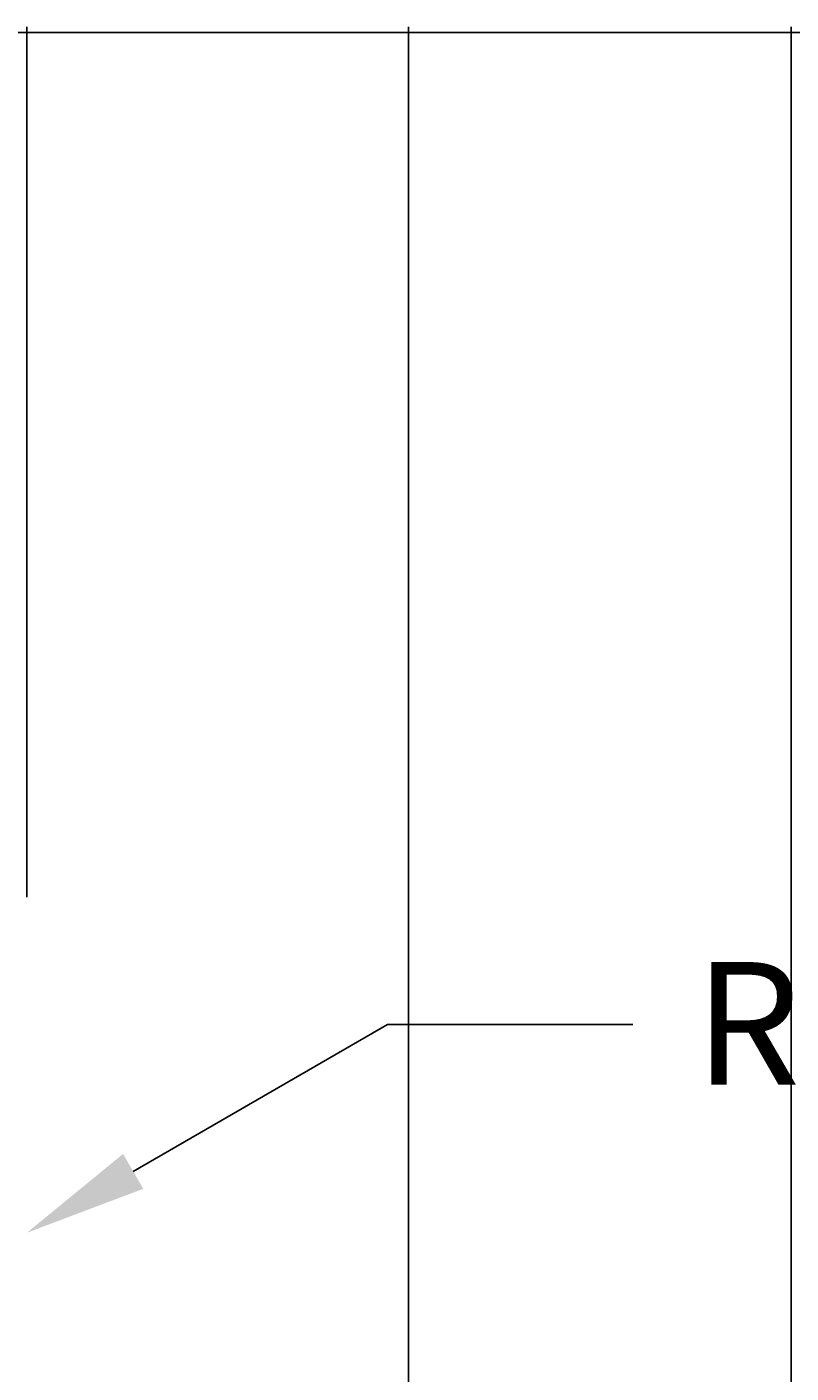
# Model space of a CAD drawing. Units: millimetres. Extents: x -11 to 280, y -4 to 208.
# Tile 18 of 55: x 66 to 91, y 164 to 208. Entities that reach past the tile are written whole.
import ezdxf
from ezdxf import colors
from ezdxf.entities.mleader import LeaderData, LeaderLine
from ezdxf.math import Vec2, Vec3

# ---------------------------------------------------------------- set-up
doc = ezdxf.new("R2010")
doc.units = ezdxf.units.MM
doc.layers.add('M-ANNO-TEXT', color=7, linetype='Continuous', lineweight=18)
doc.layers.add('M-DIMS', color=2, linetype='Continuous', lineweight=18)
doc.styles.get("Standard").update_dxf_attribs({"font": 'arial.ttf'})
doc.dimstyles.get("Standard").update_dxf_attribs({"dimtxt": 0.18, "dimasz": 0.18, "dimexe": 0.18, "dimexo": 0.0625, "dimgap": 0.09, "dimtad": 0, "dimtih": 1, "dimtoh": 1, "dimdec": 4, "dimzin": 0, "dimdsep": 46, "dimtxsty": 'Standard', "dimcen": 0.09, "dimadec": 0, "dimazin": 0, "dimtfac": 1, "dimtdec": 4, "dimtofl": 0, "dimtmove": 0, "dimatfit": 3, "dimfxl": 1, "dimtolj": 1, "dimtzin": 0, "dimarcsym": 0})

# ---------------------------------------------------------------- blocks, each defined once
blk = doc.blocks.new('*D5')
at = {"layer": 'Defpoints', "color": 0, "transparency": 16777216}
for p in [(24.759, 192.645), (-10.087, 11.435), (261.686, 11.435)]:
    blk.add_point(p, dxfattribs=at)
at = {"layer": 'M-DIMS', "color": 0, "lineweight": -2, "transparency": 16777216}
for p, q in [((24.696, 192.645), (-10.267, 192.645)), ((-10.087, 192.465), (-10.087, 102.222)), ((-10.087, 11.615), (-10.087, 101.858)), ((261.624, 11.435), (-10.267, 11.435))]:
    blk.add_line(p, q, dxfattribs=at)
at = {"layer": 'M-DIMS', "color": 0, "transparency": 16777216}
for points in [[(-10.117, 192.465), (-10.057, 192.465), (-10.087, 192.645)], [(-10.117, 11.615), (-10.057, 11.615), (-10.087, 11.435)]]:
    blk.add_solid(points, dxfattribs=at)
at = {"layer": 'M-DIMS', "color": 0, "transparency": 16777216, "insert": (-10.087, 102.04), "char_height": 0.18, "attachment_point": 5}
blk.add_mtext('\\A1;181.2', dxfattribs=at)
blk = doc.blocks.new('*D6')
at = {"layer": 'Defpoints', "color": 0, "transparency": 16777216}
for p in [(236.935, 207.495), (66.388, 179.241), (236.935, 165.103)]:
    blk.add_point(p, dxfattribs=at)
at = {"layer": 'M-DIMS', "color": 0, "lineweight": -2, "transparency": 16777216}
for p, q in [((66.388, 179.304), (66.388, 207.675)), ((236.935, 165.166), (236.935, 207.675)), ((66.568, 207.495), (151.206, 207.495)), ((236.755, 207.495), (152.117, 207.495))]:
    blk.add_line(p, q, dxfattribs=at)
at = {"layer": 'M-DIMS', "color": 0, "transparency": 16777216}
for points in [[(66.568, 207.525), (66.568, 207.465), (66.388, 207.495)], [(236.755, 207.525), (236.755, 207.465), (236.935, 207.495)]]:
    blk.add_solid(points, dxfattribs=at)
at = {"layer": 'M-DIMS', "color": 0, "transparency": 16777216, "insert": (151.661, 207.495), "char_height": 0.18, "attachment_point": 5}
blk.add_mtext('\\A1;170.55', dxfattribs=at)
blk = doc.blocks.new('*D9')
at = {"layer": 'Defpoints', "color": 0, "transparency": 16777216}
for p in [(78.827, 207.495), (31.006, 98.021), (78.827, 98.149)]:
    blk.add_point(p, dxfattribs=at)
at = {"layer": 'M-DIMS', "color": 0, "lineweight": -2, "transparency": 16777216}
for p, q in [((31.006, 98.084), (31.006, 207.675)), ((78.827, 98.212), (78.827, 207.675)), ((31.186, 207.495), (54.52, 207.495)), ((78.647, 207.495), (55.313, 207.495))]:
    blk.add_line(p, q, dxfattribs=at)
at = {"layer": 'M-DIMS', "color": 0, "transparency": 16777216}
for points in [[(31.186, 207.525), (31.186, 207.465), (31.006, 207.495)], [(78.647, 207.525), (78.647, 207.465), (78.827, 207.495)]]:
    blk.add_solid(points, dxfattribs=at)
at = {"layer": 'M-DIMS', "color": 0, "transparency": 16777216, "insert": (54.917, 207.495), "char_height": 0.18, "attachment_point": 5}
blk.add_mtext('\\A1;47.82', dxfattribs=at)
blk = doc.blocks.new('*D11')
at = {"layer": 'Defpoints', "color": 0, "transparency": 16777216}
for p in [(118.514, 207.495), (91.3, 98.149), (118.514, 96.485)]:
    blk.add_point(p, dxfattribs=at)
at = {"layer": 'M-DIMS', "color": 0, "lineweight": -2, "transparency": 16777216}
for p, q in [((91.3, 98.212), (91.3, 207.675)), ((118.514, 96.547), (118.514, 207.675)), ((91.48, 207.495), (104.442, 207.495)), ((118.334, 207.495), (105.372, 207.495))]:
    blk.add_line(p, q, dxfattribs=at)
at = {"layer": 'M-DIMS', "color": 0, "transparency": 16777216}
for points in [[(91.48, 207.525), (91.48, 207.465), (91.3, 207.495)], [(118.334, 207.525), (118.334, 207.465), (118.514, 207.495)]]:
    blk.add_solid(points, dxfattribs=at)
at = {"layer": 'M-DIMS', "color": 0, "transparency": 16777216, "insert": (104.907, 207.495), "char_height": 0.18, "attachment_point": 5}
blk.add_mtext('\\A1;27.214', dxfattribs=at)

msp = doc.modelspace()

# ---------------------------------------------------------------- dimensions: what is measured, and where the dimension line sits
at = {"layer": 'M-DIMS'}
for base, p1, p2, override, picture, middle in [((78.8273, 207.495), (31.0059, 98.0213), (78.8273, 98.1491), {"dimdec": 2, "dimlfac": 1, "dimrnd": 0, "dimzin": 0, "dimdsep": 46, "dimlunit": 2}, '*D9', (54.9166, 207.495)), ((236.9353, 207.495), (66.3875, 179.2412), (236.9353, 165.103), {"dimdec": 2, "dimlfac": 1, "dimrnd": 0, "dimzin": 0, "dimdsep": 46, "dimlunit": 2}, '*D6', (151.6614, 207.495)), ((118.5137, 207.495), (91.3, 98.1491), (118.5137, 96.4849), {"dimdec": 3, "dimlfac": 1, "dimrnd": 0, "dimzin": 0, "dimdsep": 46, "dimlunit": 2}, '*D11', (104.9068, 207.495))]:
    dim = msp.add_linear_dim(base=base, p1=p1, p2=p2, dimstyle='Standard', override=override, dxfattribs=at)
    dim.commit()
    dim.dimension.update_dxf_attribs({"geometry": picture, "text_midpoint": middle})
dim = msp.add_linear_dim(base=(-10.0865, 11.4346), p1=(24.7588, 192.645), p2=(261.6863, 11.4346), angle=90, dimstyle='Standard', override={"dimdec": 1, "dimlfac": 1, "dimrnd": 0, "dimzin": 0, "dimdsep": 46, "dimlunit": 2}, dxfattribs=at)
dim.commit()
dim.dimension.update_dxf_attribs({"geometry": '*D5', "text_midpoint": (-10.0865, 102.0398)})

# ---------------------------------------------------------------- leaders
at = {"layer": 'M-ANNO-TEXT'}
ml = msp.add_multileader_mtext('Standard', dxfattribs=at)
ml.set_content('RESERVOIR', color=256)
ml.set_leader_properties()
ml.build(insert=Vec2(0, 0))
ctx = ml.context
ctx.base_point, ctx.plane_origin = Vec3(86.1452, 175.1554), Vec3(66.3875, 168.3671)
notes = []
notes.append((ctx, [(0, (1, 1, 0), (78.1452, 175.1554), (1, 0), 8, [(0, [(66.3875, 168.3671)], 0, [])])]))
ctx.mtext.insert, ctx.mtext.flow_direction = Vec3(88.1452, 177.1895), 5
for ctx, leaders in notes:
    for number, flags, end, landing, length, lines in leaders:
        leader = LeaderData()
        leader.index, (leader.has_last_leader_line, leader.has_dogleg_vector, leader.attachment_direction) = number, flags
        leader.last_leader_point, leader.dogleg_vector, leader.dogleg_length = Vec3(end), Vec3(landing), length
        for number, points, colour, breaks in lines:
            line = LeaderLine()
            line.index, line.vertices, line.color, line.breaks = number, Vec3.list(points), colors.encode_raw_color(colour), breaks
            leader.lines.append(line)
        ctx.leaders.append(leader)

doc.saveas('drawing.dxf')
